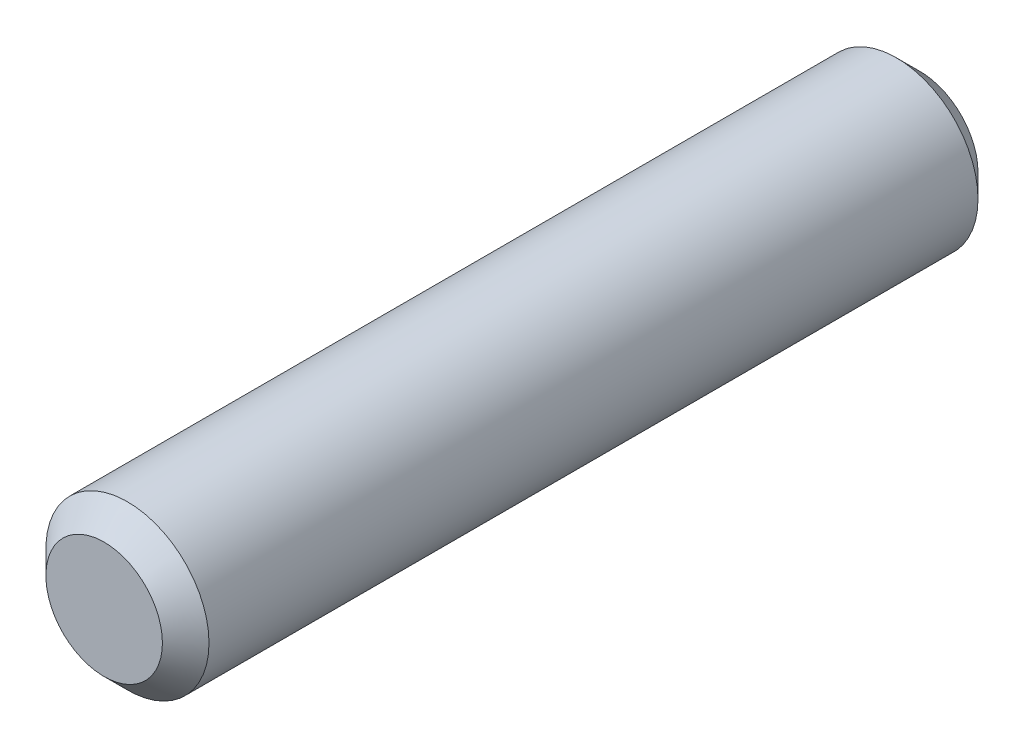
ISO-10303-21;
HEADER;
FILE_DESCRIPTION(('STEP AP214'),'2;1');
FILE_NAME('part.step','',(''),(''),'','','');
FILE_SCHEMA(('AUTOMOTIVE_DESIGN { 1 0 10303 214 1 1 1 1 }'));
ENDSEC;
DATA;
#1=APPLICATION_CONTEXT('core data for automotive mechanical design processes');
#2=APPLICATION_PROTOCOL_DEFINITION('international standard','automotive_design',2000,#1);
#3=PRODUCT_CONTEXT('',#1,'mechanical');
#4=PRODUCT('Part','Part','',(#3));
#5=PRODUCT_RELATED_PRODUCT_CATEGORY('part','',(#4));
#6=PRODUCT_DEFINITION_FORMATION('','',#4);
#7=PRODUCT_DEFINITION_CONTEXT('part definition',#1,'design');
#8=PRODUCT_DEFINITION('design','',#6,#7);
#9=PRODUCT_DEFINITION_SHAPE('','',#8);
#10=(LENGTH_UNIT() NAMED_UNIT(*) SI_UNIT(.MILLI.,.METRE.));
#11=(NAMED_UNIT(*) PLANE_ANGLE_UNIT() SI_UNIT($,.RADIAN.));
#12=(NAMED_UNIT(*) SI_UNIT($,.STERADIAN.) SOLID_ANGLE_UNIT());
#13=UNCERTAINTY_MEASURE_WITH_UNIT(LENGTH_MEASURE(1.E-05),#10,'distance_accuracy_value','');
#14=(GEOMETRIC_REPRESENTATION_CONTEXT(3) GLOBAL_UNCERTAINTY_ASSIGNED_CONTEXT((#13)) GLOBAL_UNIT_ASSIGNED_CONTEXT((#10,
#11,#12)) REPRESENTATION_CONTEXT('',''));
#15=CARTESIAN_POINT('',(0.,0.,0.));
#16=DIRECTION('',(0.,0.,1.));
#17=DIRECTION('',(1.,0.,0.));
#18=AXIS2_PLACEMENT_3D('',#15,#16,#17);
#19=CARTESIAN_POINT('',(0.,0.,35.));
#20=DIRECTION('',(0.,0.,-1.));
#21=DIRECTION('',(-1.,0.,0.));
#22=AXIS2_PLACEMENT_3D('',#19,#20,#21);
#23=CYLINDRICAL_SURFACE('',#22,7.);
#24=CARTESIAN_POINT('',(0.,0.,-33.));
#25=DIRECTION('',(0.,0.,1.));
#26=DIRECTION('',(1.,0.,0.));
#27=AXIS2_PLACEMENT_3D('',#24,#25,#26);
#28=CIRCLE('',#27,7.);
#29=CARTESIAN_POINT('',(7.,0.,-33.));
#30=VERTEX_POINT('',#29);
#31=EDGE_CURVE('E50',#30,#30,#28,.T.);
#32=ORIENTED_EDGE('',*,*,#31,.T.);
#33=EDGE_LOOP('',(#32));
#34=FACE_BOUND('',#33,.T.);
#35=CARTESIAN_POINT('',(0.,0.,33.));
#36=DIRECTION('',(0.,0.,1.));
#37=DIRECTION('',(1.,0.,0.));
#38=AXIS2_PLACEMENT_3D('',#35,#36,#37);
#39=CIRCLE('',#38,7.);
#40=CARTESIAN_POINT('',(7.,0.,33.));
#41=VERTEX_POINT('',#40);
#42=EDGE_CURVE('E51',#41,#41,#39,.F.);
#43=ORIENTED_EDGE('',*,*,#42,.T.);
#44=EDGE_LOOP('',(#43));
#45=FACE_BOUND('',#44,.T.);
#46=ADVANCED_FACE('F39',(#34,#45),#23,.T.);
#47=CARTESIAN_POINT('',(0.,0.,35.));
#48=DIRECTION('',(0.,0.,1.));
#49=DIRECTION('',(1.,0.,0.));
#50=AXIS2_PLACEMENT_3D('',#47,#48,#49);
#51=PLANE('',#50);
#52=CARTESIAN_POINT('',(0.,0.,35.));
#53=DIRECTION('',(0.,0.,1.));
#54=DIRECTION('',(1.,0.,0.));
#55=AXIS2_PLACEMENT_3D('',#52,#53,#54);
#56=CIRCLE('',#55,4.99999999999998);
#57=CARTESIAN_POINT('',(4.99999999999998,0.,35.));
#58=VERTEX_POINT('',#57);
#59=EDGE_CURVE('E54',#58,#58,#56,.T.);
#60=ORIENTED_EDGE('',*,*,#59,.T.);
#61=EDGE_LOOP('',(#60));
#62=FACE_BOUND('',#61,.T.);
#63=ADVANCED_FACE('F61',(#62),#51,.T.);
#64=CARTESIAN_POINT('',(0.,0.,-35.));
#65=DIRECTION('',(0.,0.,1.));
#66=DIRECTION('',(1.,0.,0.));
#67=AXIS2_PLACEMENT_3D('',#64,#65,#66);
#68=PLANE('',#67);
#69=CARTESIAN_POINT('',(0.,0.,-35.));
#70=DIRECTION('',(0.,0.,1.));
#71=DIRECTION('',(1.,0.,0.));
#72=AXIS2_PLACEMENT_3D('',#69,#70,#71);
#73=CIRCLE('',#72,4.99999999999999);
#74=CARTESIAN_POINT('',(4.99999999999999,0.,-35.));
#75=VERTEX_POINT('',#74);
#76=EDGE_CURVE('E10',#75,#75,#73,.F.);
#77=ORIENTED_EDGE('',*,*,#76,.T.);
#78=EDGE_LOOP('',(#77));
#79=FACE_BOUND('',#78,.T.);
#80=ADVANCED_FACE('F64',(#79),#68,.F.);
#81=CARTESIAN_POINT('',(0.,0.,35.));
#82=DIRECTION('',(0.,0.,-1.));
#83=DIRECTION('',(-1.,0.,0.));
#84=AXIS2_PLACEMENT_3D('',#81,#82,#83);
#85=CONICAL_SURFACE('',#84,4.99999999999998,0.785398163397445);
#86=ORIENTED_EDGE('',*,*,#42,.F.);
#87=EDGE_LOOP('',(#86));
#88=FACE_BOUND('',#87,.T.);
#89=ORIENTED_EDGE('',*,*,#59,.F.);
#90=EDGE_LOOP('',(#89));
#91=FACE_BOUND('',#90,.T.);
#92=ADVANCED_FACE('F62',(#88,#91),#85,.T.);
#93=CARTESIAN_POINT('',(0.,0.,-33.));
#94=DIRECTION('',(0.,0.,1.));
#95=DIRECTION('',(1.,0.,0.));
#96=AXIS2_PLACEMENT_3D('',#93,#94,#95);
#97=CONICAL_SURFACE('',#96,7.,0.78539816339745);
#98=ORIENTED_EDGE('',*,*,#76,.F.);
#99=EDGE_LOOP('',(#98));
#100=FACE_BOUND('',#99,.T.);
#101=ORIENTED_EDGE('',*,*,#31,.F.);
#102=EDGE_LOOP('',(#101));
#103=FACE_BOUND('',#102,.T.);
#104=ADVANCED_FACE('F45',(#100,#103),#97,.T.);
#105=CLOSED_SHELL('',(#46,#63,#80,#92,#104));
#106=MANIFOLD_SOLID_BREP('B2',#105);
#107=ADVANCED_BREP_SHAPE_REPRESENTATION('',(#18,#106),#14);
#108=SHAPE_DEFINITION_REPRESENTATION(#9,#107);
ENDSEC;
END-ISO-10303-21;
